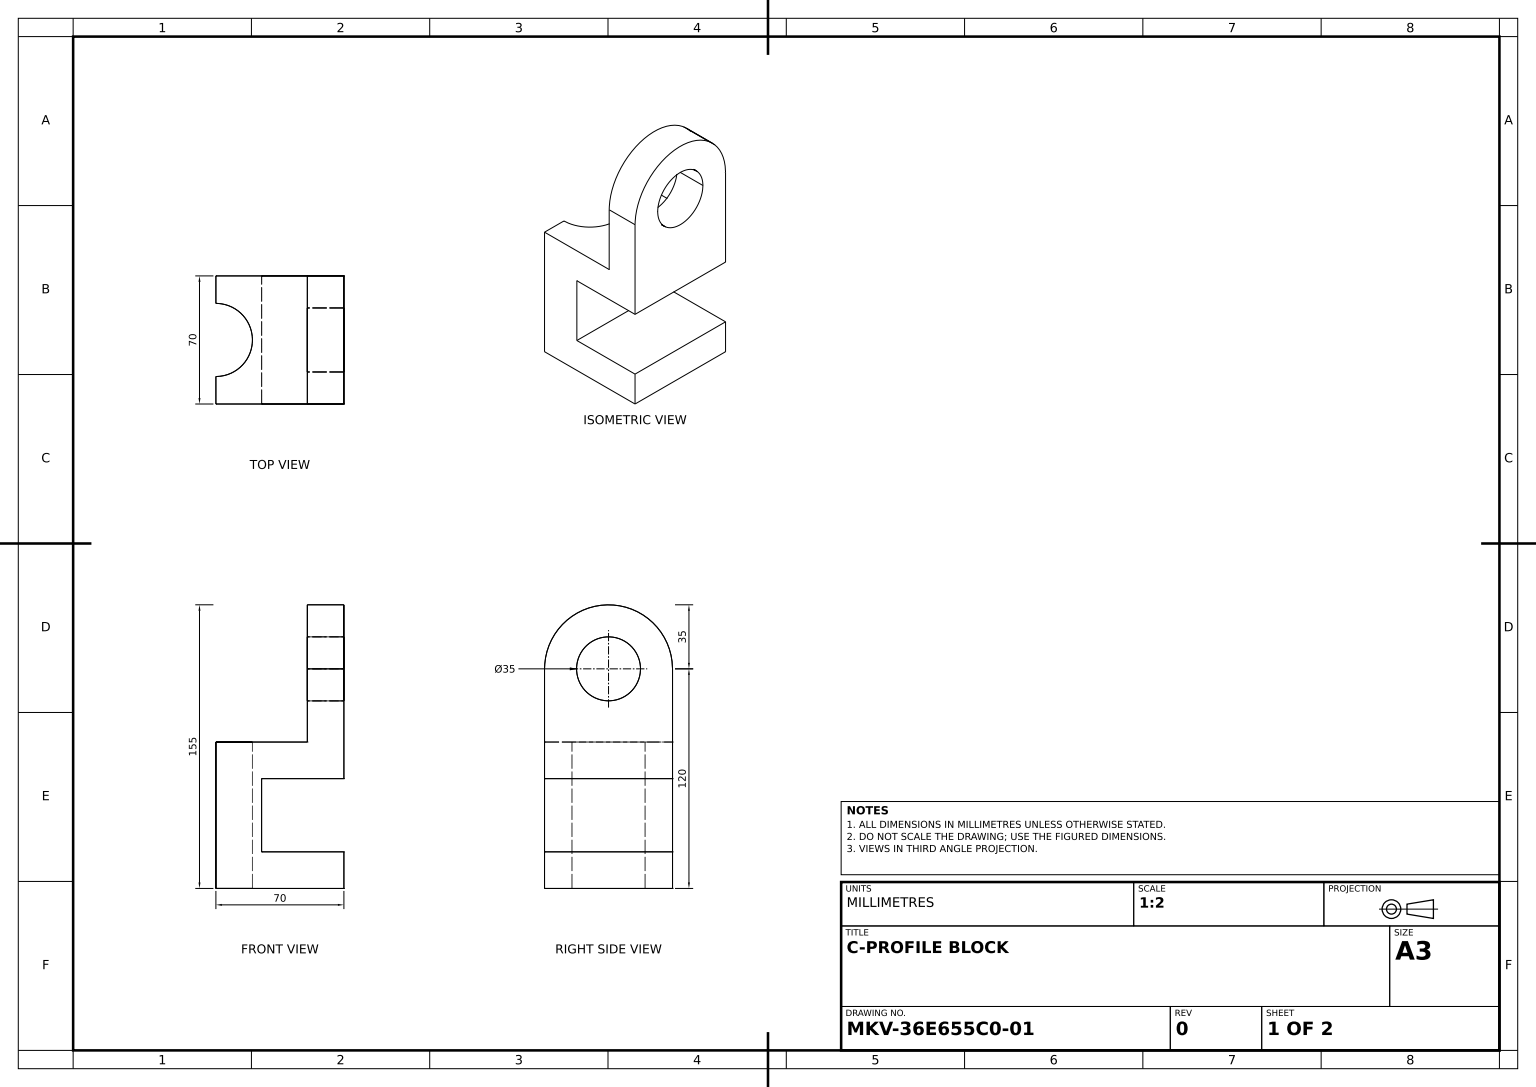
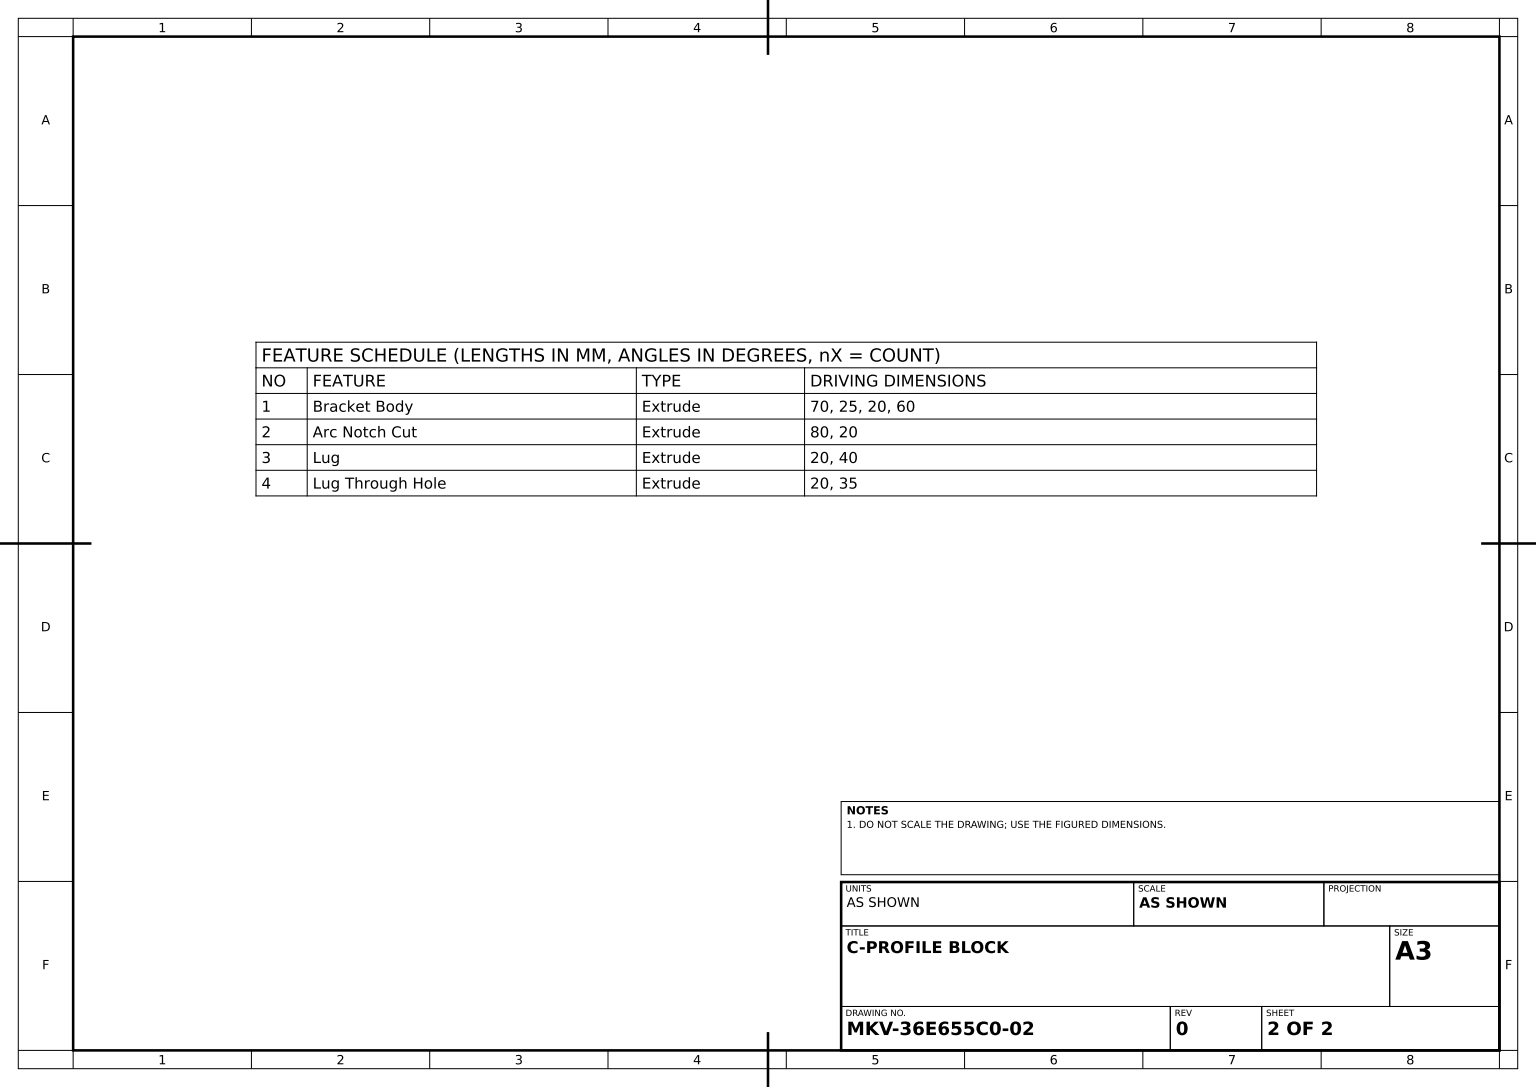
SolidWorks part; units mm, degrees
material "Plain Carbon Steel"
ref_plane "Front Plane" through (0, 0, 0) normal (0, 0, 1) x (1, 0, 0)
ref_plane "Top Plane" through (0, 0, 0) normal (0, 1, 0) x (1, 0, 0)
ref_plane "Right Plane" through (0, 0, 0) normal (1, 0, 0) x (0, 0, -1)
sketch "Bracket Profile Sketch" plane through (0, 0, 0) normal (0, 0, 1) x (1, 0, 0)
  line L0 (0, 0) -> (70, 0)
  line L1 (70, 0) -> (70, 20)
  line L2 (70, 20) -> (25, 20)
  line L3 (25, 20) -> (25, 60)
  line L4 (25, 60) -> (70, 60)
  line L5 (70, 60) -> (70, 80)
  line L6 (70, 80) -> (0, 80)
  line L7 (0, 80) -> (0, 0)
  dimension "D1" = 25
  dimension "D2" = 70
  dimension "D3" = 20
  dimension "D4" = 60
extrude "Bracket Body" add sketch "Bracket Profile Sketch" along normal blind 70
sketch "Arc Notch Sketch" plane through (0, 80, 0) normal (0, 1, 0) x (1, 0, 0)
  line L0 (0, -70) -> (0, 0) construction
  line L1 (0, -15) -> (0, -55)
  arc A0 (0, -55) -> (0, -15) centre (0, -35) ccw
  dimension "D1" = 20
extrude "Arc Notch Cut" cut sketch "Arc Notch Sketch" against normal blind 80
sketch "Lug Profile Sketch" plane through (70, 0, 0) normal (1, 0, 0) x (0, 0, -1)
  line L1 (-70, 80) -> (0, 80) construction
  line L2 (-70, 120) -> (-70, 80)
  line L3 (-70, 80) -> (0, 80)
  line L4 (0, 80) -> (0, 120)
  arc A0 (0, 120) -> (-70, 120) centre (-35, 120) ccw
  dimension "D1" = 40
extrude "Lug" add sketch "Lug Profile Sketch" against normal blind 20
sketch "Lug Hole Sketch" plane through (50, 0, 0) normal (-1, 0, 0) x (0, 0, 1)
  circle A0 centre (35, 120) radius 17.5
  dimension "D1" = 35
  dimension "D2" = 35
extrude "Lug Through Hole" cut sketch "Lug Hole Sketch" against normal blind 20
